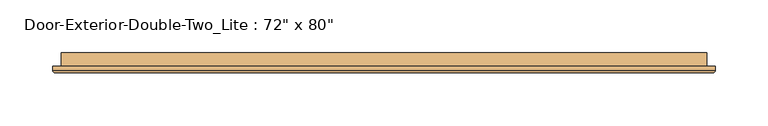
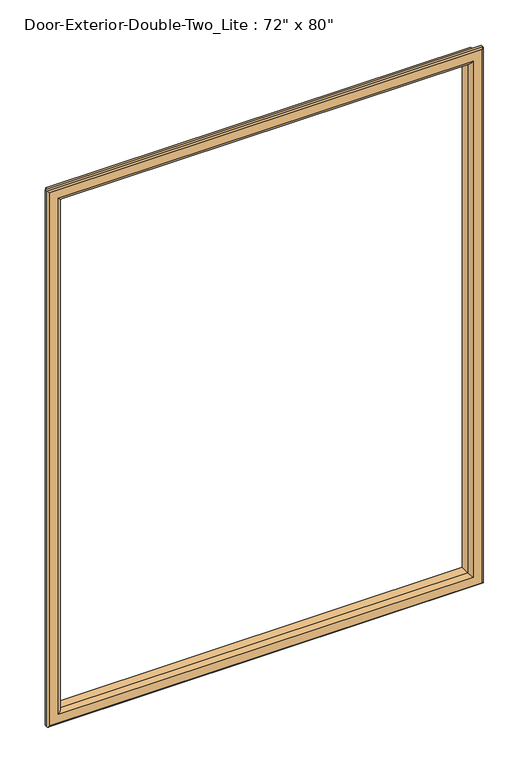
"""IFC4 building model written with IfcOpenShell, lengths in millimetres: door geometry."""

from ifc_helpers import new_model, si_unit, frame, origin, place, context, project, spatial, ellipse_curve, source, transform, mapped, element, save
from ifc_brep_helpers import plane_surface, cylinder_surface, advanced_brep


def door_2f28d345(model_context):
    return source(origin(), model_context, "Body", "AdvancedBrep", [
        advanced_brep(
        [(-762.0, 50.8, 1117.6), (-762.0, 38.1, 1117.6), (-762.0, 38.1, 1914.525), (-762.0, 50.8, 1914.525), (-750.0, 37.1, 1129.6), (-750.0, 50.8, 1129.6), (-750.0, 50.8, 1902.525), (-750.0, 37.1, 1902.525), (-755.0, 32.1, 1124.6), (-755.0, 32.1, 1907.525), (-770.0, 34.1, 1109.6), (-768.0, 32.1, 1111.6), (-768.0, 32.1, 1920.525), (-770.0, 34.1, 1922.525), (-770.0, 38.1, 1109.6), (-770.0, 38.1, 1922.525), (-152.4, 38.1, 1914.525), (-152.4, 50.8, 1914.525), (-164.4, 50.8, 1902.525), (-164.4, 37.1, 1902.525), (-159.4, 32.1, 1907.525), (-146.4, 32.1, 1920.525), (-144.4, 34.1, 1922.525), (-144.4, 38.1, 1922.525), (-152.4, 38.1, 1117.6), (-152.4, 50.8, 1117.6), (-164.4, 50.8, 1129.6), (-164.4, 37.1, 1129.6), (-159.4, 32.1, 1124.6), (-146.4, 32.1, 1111.6), (-144.4, 34.1, 1109.6), (-144.4, 38.1, 1109.6)],
        [
            (0, 1),
            (1, 2),
            (2, 3),
            (3, 0),
            (4, 5),
            (5, 6),
            (6, 7),
            (7, 4),
            (8, 4, ellipse_curve(frame((-755.0, 37.1, 1124.6), z_axis=(-0.7071067811865475, 0.0, 0.7071067811865475), x_axis=(-0.7071067811865474, 0.0, -0.7071067811865476)), 7.0710678, 5.0)),
            (7, 9, ellipse_curve(frame((-755.0, 37.1, 1907.525), z_axis=(-0.7071067811865475, 0.0, -0.7071067811865475), x_axis=(0.7071067811865474, 0.0, -0.7071067811865476)), 7.0710678, 5.0)),
            (9, 8),
            (10, 11, ellipse_curve(frame((-768.0, 34.1, 1111.6), z_axis=(-0.7071067811865475, 0.0, 0.7071067811865475), x_axis=(-0.7071067811865474, 0.0, -0.7071067811865476)), 2.8284271, 2.0)),
            (11, 12),
            (12, 13, ellipse_curve(frame((-768.0, 34.1, 1920.525), z_axis=(-0.7071067811865475, 0.0, -0.7071067811865475), x_axis=(0.7071067811865474, 0.0, -0.7071067811865476)), 2.8284271, 2.0)),
            (13, 10),
            (14, 10),
            (13, 15),
            (15, 14),
            (2, 16),
            (16, 17),
            (17, 3),
            (6, 18),
            (18, 19),
            (19, 7),
            (19, 20, ellipse_curve(frame((-159.4, 37.1, 1907.525), z_axis=(-0.7071067811865475, 0.0, 0.7071067811865475), x_axis=(-0.7071067811865476, 0.0, -0.7071067811865474)), 7.0710678, 5.0)),
            (20, 9),
            (12, 21),
            (21, 22, ellipse_curve(frame((-146.4, 34.1, 1920.525), z_axis=(-0.7071067811865475, 0.0, 0.7071067811865475), x_axis=(-0.7071067811865476, 0.0, -0.7071067811865474)), 2.8284271, 2.0)),
            (22, 13),
            (22, 23),
            (23, 15),
            (16, 24),
            (24, 25),
            (25, 17),
            (18, 26),
            (26, 27),
            (27, 19),
            (27, 28, ellipse_curve(frame((-159.4, 37.1, 1124.6), z_axis=(0.7071067811865475, 0.0, 0.7071067811865475), x_axis=(-0.7071067811865474, 0.0, 0.7071067811865476)), 7.0710678, 5.0)),
            (28, 20),
            (21, 29),
            (29, 30, ellipse_curve(frame((-146.4, 34.1, 1111.6), z_axis=(0.7071067811865475, 0.0, 0.7071067811865475), x_axis=(-0.7071067811865474, 0.0, 0.7071067811865476)), 2.8284271, 2.0)),
            (30, 22),
            (30, 31),
            (31, 23),
            (31, 14),
            (1, 24),
            (0, 25),
            (5, 26),
            (4, 27),
            (8, 28),
            (11, 29),
            (10, 30),
        ],
        [
            plane_surface(frame((-762.0, 38.1, 1117.6), z_axis=(-1.0, 0.0, 0.0), x_axis=(0.0, 0.0, 1.0))),
            plane_surface(frame((-750.0, 50.8, 1129.6), z_axis=(1.0, 0.0, 0.0), x_axis=(0.0, 0.0, 1.0))),
            cylinder_surface(frame((-755.0, 37.1, 1117.6), z_axis=(0.0, 0.0, -1.0), x_axis=(-1.0, 0.0, 0.0)), 5.0),
            cylinder_surface(frame((-768.0, 34.1, 1117.6), z_axis=(0.0, 0.0, -1.0), x_axis=(-1.0, 0.0, 0.0)), 2.0),
            plane_surface(frame((-770.0, 34.1, 1109.6), z_axis=(-1.0, 0.0, 0.0), x_axis=(0.0, 0.0, 1.0))),
            plane_surface(frame((-762.0, 38.1, 1914.525), z_axis=(0.0, 0.0, 1.0), x_axis=(1.0, 0.0, 0.0))),
            plane_surface(frame((-750.0, 50.8, 1902.525), z_axis=(0.0, 0.0, -1.0), x_axis=(1.0, 0.0, 0.0))),
            cylinder_surface(frame((-762.0, 37.1, 1907.525), z_axis=(-1.0, 0.0, 0.0), x_axis=(0.0, 0.0, 1.0)), 5.0),
            cylinder_surface(frame((-762.0, 34.1, 1920.525), z_axis=(-1.0, 0.0, 0.0), x_axis=(0.0, 0.0, 1.0)), 2.0),
            plane_surface(frame((-770.0, 34.1, 1922.525), z_axis=(0.0, 0.0, 1.0), x_axis=(1.0, 0.0, 0.0))),
            plane_surface(frame((-152.4, 38.1, 1914.525), z_axis=(1.0, 0.0, 0.0), x_axis=(0.0, 0.0, -1.0))),
            plane_surface(frame((-164.4, 50.8, 1902.525), z_axis=(-1.0, 0.0, 0.0), x_axis=(0.0, 0.0, -1.0))),
            cylinder_surface(frame((-159.4, 37.1, 1914.525), z_axis=(0.0, 0.0, 1.0), x_axis=(1.0, 0.0, 0.0)), 5.0),
            cylinder_surface(frame((-146.4, 34.1, 1914.525), z_axis=(0.0, 0.0, 1.0), x_axis=(1.0, 0.0, 0.0)), 2.0),
            plane_surface(frame((-144.4, 34.1, 1922.525), z_axis=(1.0, 0.0, 0.0), x_axis=(0.0, 0.0, -1.0))),
            plane_surface(frame((-144.4, 38.1, 1109.6), z_axis=(0.0, 1.0, 0.0), x_axis=(-1.0, 0.0, 0.0))),
            plane_surface(frame((-152.4, 38.1, 1117.6), z_axis=(0.0, 0.0, -1.0), x_axis=(-1.0, 0.0, 0.0))),
            plane_surface(frame((-152.4, 50.8, 1117.6), z_axis=(0.0, 1.0, 0.0), x_axis=(-1.0, 0.0, 0.0))),
            plane_surface(frame((-164.4, 50.8, 1129.6), z_axis=(0.0, 0.0, 1.0), x_axis=(-1.0, 0.0, 0.0))),
            cylinder_surface(frame((-152.4, 37.1, 1124.6), z_axis=(1.0, 0.0, 0.0), x_axis=(0.0, 0.0, -1.0)), 5.0),
            plane_surface(frame((-159.4, 32.1, 1124.6), z_axis=(0.0, -1.0, 0.0), x_axis=(-1.0, 0.0, 0.0))),
            cylinder_surface(frame((-152.4, 34.1, 1111.6), z_axis=(1.0, 0.0, 0.0), x_axis=(0.0, 0.0, -1.0)), 2.0),
            plane_surface(frame((-144.4, 34.1, 1109.6), z_axis=(0.0, 0.0, -1.0), x_axis=(-1.0, 0.0, 0.0))),
        ],
        [
            (0, [[1, 2, 3, 4]]),
            (1, [[5, 6, 7, 8]]),
            (2, [[9, -8, 10, 11]]),
            (3, [[12, 13, 14, 15]]),
            (4, [[16, -15, 17, 18]]),
            (5, [[-3, 19, 20, 21]]),
            (6, [[-7, 22, 23, 24]]),
            (7, [[-10, -24, 25, 26]]),
            (8, [[-14, 27, 28, 29]]),
            (9, [[-17, -29, 30, 31]]),
            (10, [[-20, 32, 33, 34]]),
            (11, [[-23, 35, 36, 37]]),
            (12, [[-25, -37, 38, 39]]),
            (13, [[-28, 40, 41, 42]]),
            (14, [[-30, -42, 43, 44]]),
            (15, [[-31, -44, 45, -18], [46, -32, -19, -2]]),
            (16, [[-33, -46, -1, 47]]),
            (17, [[-21, -34, -47, -4], [48, -35, -22, -6]]),
            (18, [[-36, -48, -5, 49]]),
            (19, [[-38, -49, -9, 50]]),
            (20, [[51, -40, -27, -13], [-26, -39, -50, -11]]),
            (21, [[-41, -51, -12, 52]]),
            (22, [[-43, -52, -16, -45]]),
        ],
    ),
    ])


if __name__ == "__main__":
    model = new_model("IFC4")
    model_context = context("Model", 3, world=origin())
    ifc_project = project(units=[si_unit("LENGTHUNIT", "METRE", prefix="MILLI")], contexts=[model_context])
    site = spatial("IfcSite", under=ifc_project)
    building = spatial("IfcBuilding", under=site)
    placement = place(None, origin())
    door_shape = door_2f28d345(model_context)
    element("IfcDoor", 1, ObjectType="Door-Exterior-Double-Two_Lite : 72\" x 80\"", at=placement, inside=building, context=model_context, shape_type="MappedRepresentation", body=[
        mapped(door_shape, transform((0.0, 0.0, 0.0), x_axis=(1.0, 0.0, 0.0), y_axis=(0.0, 1.0, 0.0), z_axis=(0.0, 0.0, 1.0))),
    ])
    save(model, "model.ifc")

# Revit data of these elements
# Type "Door-Exterior-Double-Two_Lite : 72\" x 80\""
#   Type Mark = "10"
#   Assembly Code = "B2030100"
#   Analytic Construction = "Metal frame, double glass door"
#   Top Rail = 0' - 4 5/8"
#   Threshold Length [instance default] = 6' - 4"
#   Threshold Offset [instance default] = 0' - 0 1/2"
#   Thickness = 0' - 1 3/4"
#   Thermal Resistance (R) = 1.3794 (h·ft²·°F)/BTU
#   Swing Angle [instance default] = 90.00°
#   Strike Height = 3' - 4"
#   Stiles = 0' - 6"
#   SinglePanelWidth = 3' - 0"
#   Rough Width [instance default] = 6' - 4"
#   Rough Height [instance default] = 7' - 0"
#   MFOpeningHeight [instance default] = 0' - 4"
#   MFOpeningWidth [instance default] = 0' - 4"
#   Lock Rail = 0' - 8"
#   Inset Calculate [instance default] = 0' - 4"
#   Masonry Inset [instance default] = 0' - 1"
#   Height = 6' - 8"
#   Width = 6' - 0"
#   Heat Transfer Coefficient (U) = 0.7250 BTU/(h·ft²·°F)
#   Glass Thickness = 0' - 0 3/4"
#   Masonry Frame Depth = 0' - 5 3/4"
#   Bottom Rail = 0' - 10"
#   Threshold [instance default] = yes
#   Masonry Frame [instance default] = yes
#   Function = 1
#   Dry Wall Frame [instance default] = no
#   Threshold Material = none
#   Panic Bar Material = Metal - Stainless Steel
#   Panel Material = Metal - Painted - Grey
#   Glass Stop Material = Metal - Painted - Grey
#   Frame Material = Metal - Painted - Grey
#   Exterior Pull Material = Metal - Stainless Steel
#   Visual Light Transmittance = 0
#   Solar Heat Gain Coefficient = 0
#   Wall Closure = (empty or 0)
# Element 1 (IfcDoor, "Door-Exterior-Double-Two_Lite : 72\" x 80\"")
#   Materials on its faces: "Metal - Painted - Grey", "Metal - Stainless Steel", "Glass"
# Materials
#   "Metal - Stainless Steel": class "Metal", colour RGB 247 247 247, transparency 0
#   "Metal - Painted - Grey": class "Paint", colour RGB 104 104 104, transparency 0, Cost = 0
#   "Glass": class "Glass", colour RGB 0 128 192, transparency 0.75, Description = "Soda Lime Glass", Cost = 0
